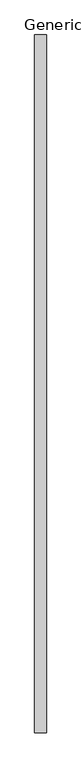
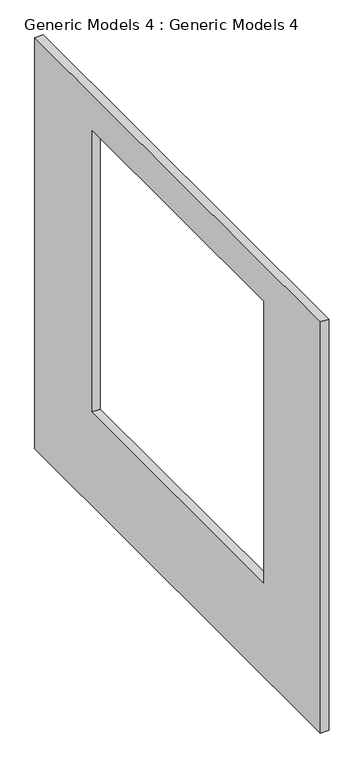
"""IFC4 building model written with IfcOpenShell, lengths in millimetres: proxy geometry, Generic Models 4 : Generic Models 4."""

from ifc_helpers import new_model, si_unit, frame, origin, place, context, project, spatial, polyline, outline, extrude, source, transform, mapped, element, save


def generic_models_4_generic_models_4_9c707661(model_context):
    return source(origin(), model_context, "Body", "SweptSolid", [
        extrude(outline(polyline([(4102.1641252, 3014.1333333), (4102.1641252, 339.6), (1054.1641252, 339.6), (1054.1641252, 3014.1333333), (4102.1641252, 3014.1333333)]), holes=[polyline([(3492.5641252, 2778.0), (1663.7641252, 2778.0), (1663.7641252, 949.2), (3492.5641252, 949.2), (3492.5641252, 2778.0)])]), frame((4189.5719693, 0.0, 0.0), z_axis=(1.0, 0.0, 0.0), x_axis=(0.0, 1.0, 0.0)), (0.0, 0.0, 1.0), 50.8),
    ])


if __name__ == "__main__":
    model = new_model("IFC4")
    model_context = context("Model", 3, world=origin())
    ifc_project = project(units=[si_unit("LENGTHUNIT", "METRE", prefix="MILLI")], contexts=[model_context])
    site = spatial("IfcSite", under=ifc_project)
    building = spatial("IfcBuilding", under=site)
    placement = place(None, origin())
    generic_models_4_generic_models_4_shape = generic_models_4_generic_models_4_9c707661(model_context)
    element("IfcBuildingElementProxy", 1, Name="Generic Models 4 : Generic Models 4", ObjectType="Generic Models 4 : Generic Models 4", at=placement, inside=building, context=model_context, shape_type="MappedRepresentation", body=[
        mapped(generic_models_4_generic_models_4_shape, transform((0.0, 0.0, 0.0), x_axis=(1.0, 0.0, 0.0), y_axis=(0.0, 1.0, 0.0), z_axis=(0.0, 0.0, 1.0))),
    ])
    save(model, "model.ifc")
